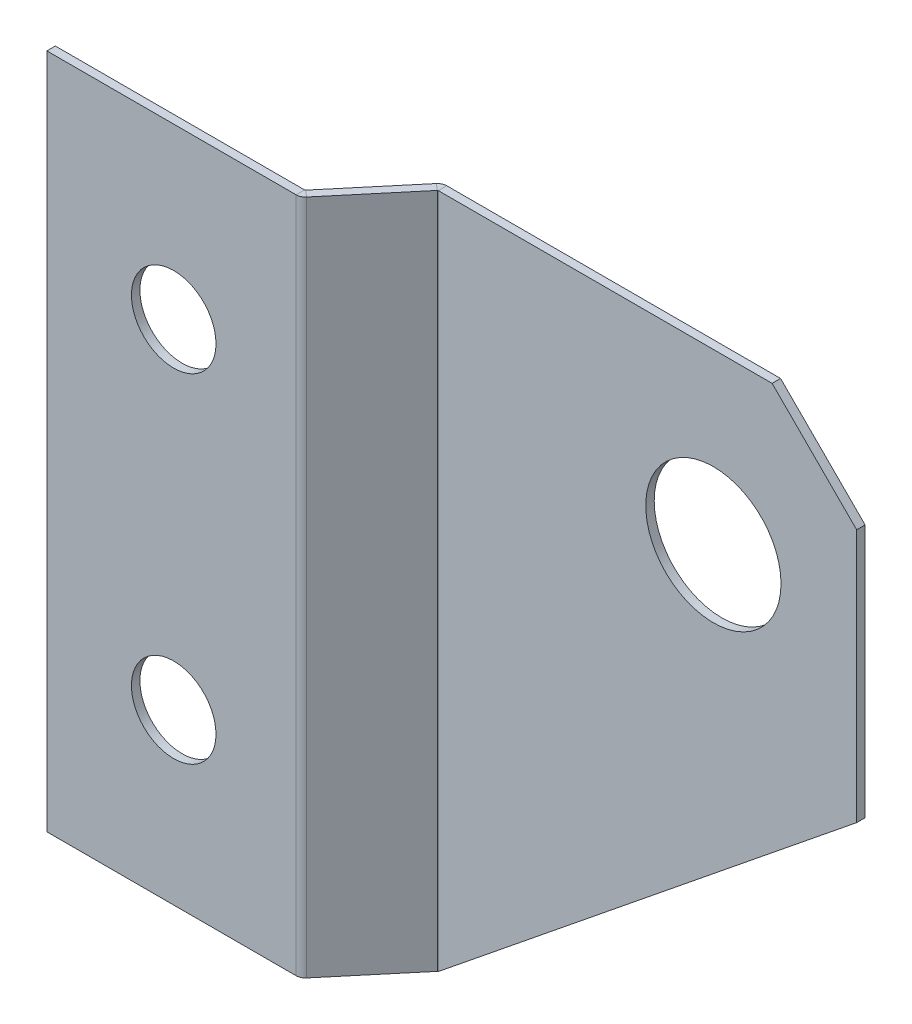
ISO-10303-21;
HEADER;
FILE_DESCRIPTION(('STEP AP214'),'2;1');
FILE_NAME('part.step','',(''),(''),'','','');
FILE_SCHEMA(('AUTOMOTIVE_DESIGN { 1 0 10303 214 1 1 1 1 }'));
ENDSEC;
DATA;
#1=APPLICATION_CONTEXT('core data for automotive mechanical design processes');
#2=APPLICATION_PROTOCOL_DEFINITION('international standard','automotive_design',2000,#1);
#3=PRODUCT_CONTEXT('',#1,'mechanical');
#4=PRODUCT('Part','Part','',(#3));
#5=PRODUCT_RELATED_PRODUCT_CATEGORY('part','',(#4));
#6=PRODUCT_DEFINITION_FORMATION('','',#4);
#7=PRODUCT_DEFINITION_CONTEXT('part definition',#1,'design');
#8=PRODUCT_DEFINITION('design','',#6,#7);
#9=PRODUCT_DEFINITION_SHAPE('','',#8);
#10=(LENGTH_UNIT() NAMED_UNIT(*) SI_UNIT(.MILLI.,.METRE.));
#11=(NAMED_UNIT(*) PLANE_ANGLE_UNIT() SI_UNIT($,.RADIAN.));
#12=(NAMED_UNIT(*) SI_UNIT($,.STERADIAN.) SOLID_ANGLE_UNIT());
#13=UNCERTAINTY_MEASURE_WITH_UNIT(LENGTH_MEASURE(1.E-05),#10,'distance_accuracy_value','');
#14=(GEOMETRIC_REPRESENTATION_CONTEXT(3) GLOBAL_UNCERTAINTY_ASSIGNED_CONTEXT((#13)) GLOBAL_UNIT_ASSIGNED_CONTEXT((#10,
#11,#12)) REPRESENTATION_CONTEXT('',''));
#15=CARTESIAN_POINT('',(0.,0.,0.));
#16=DIRECTION('',(0.,0.,1.));
#17=DIRECTION('',(1.,0.,0.));
#18=AXIS2_PLACEMENT_3D('',#15,#16,#17);
#19=CARTESIAN_POINT('',(3.85672565811926,40.,-4.59626665871385));
#20=DIRECTION('',(0.,1.,0.));
#21=DIRECTION('',(0.,0.,1.));
#22=AXIS2_PLACEMENT_3D('',#19,#20,#21);
#23=PLANE('',#22);
#24=DIRECTION('',(0.642787609686543,0.,-0.766044443118975));
#25=VECTOR('',#24,1.);
#26=CARTESIAN_POINT('',(3.85672565811926,40.,-4.59626665871385));
#27=LINE('',#26,#25);
#28=CARTESIAN_POINT('',(0.164855231730187,40.,-0.196466814672401));
#29=VERTEX_POINT('',#28);
#30=CARTESIAN_POINT('',(3.69187042638907,40.,-4.39979984404145));
#31=VERTEX_POINT('',#30);
#32=EDGE_CURVE('E239',#29,#31,#27,.T.);
#33=ORIENTED_EDGE('',*,*,#32,.T.);
#34=DIRECTION('',(-0.766044443118972,0.,-0.642787609686546));
#35=VECTOR('',#34,1.);
#36=CARTESIAN_POINT('',(3.69187042638907,40.,-4.39979984404145));
#37=LINE('',#36,#35);
#38=CARTESIAN_POINT('',(3.30884820482958,40.,-4.72119364888472));
#39=VERTEX_POINT('',#38);
#40=EDGE_CURVE('E218',#31,#39,#37,.T.);
#41=ORIENTED_EDGE('',*,*,#40,.T.);
#42=DIRECTION('',(-0.642787609686543,0.,0.766044443118975));
#43=VECTOR('',#42,1.);
#44=CARTESIAN_POINT('',(-0.479355767330552,40.,-0.20658795558327));
#45=LINE('',#44,#43);
#46=CARTESIAN_POINT('',(-0.218166989829301,40.,-0.517860619515672));
#47=VERTEX_POINT('',#46);
#48=EDGE_CURVE('E244',#47,#39,#45,.F.);
#49=ORIENTED_EDGE('',*,*,#48,.F.);
#50=DIRECTION('',(0.766044443118975,0.,0.642787609686543));
#51=VECTOR('',#50,1.);
#52=CARTESIAN_POINT('',(0.164855231730188,40.,-0.1964668146724));
#53=LINE('',#52,#51);
#54=EDGE_CURVE('E232',#47,#29,#53,.T.);
#55=ORIENTED_EDGE('',*,*,#54,.T.);
#56=EDGE_LOOP('',(#33,#41,#49,#55));
#57=FACE_BOUND('',#56,.T.);
#58=ADVANCED_FACE('F83',(#57),#23,.T.);
#59=CARTESIAN_POINT('',(-0.0963335457710638,0.,0.114805849260002));
#60=DIRECTION('',(0.766044443118975,0.,0.642787609686543));
#61=DIRECTION('',(0.642787609686543,0.,-0.766044443118975));
#62=AXIS2_PLACEMENT_3D('',#59,#60,#61);
#63=PLANE('',#62);
#64=DIRECTION('',(-0.642787609686543,0.,0.766044443118975));
#65=VECTOR('',#64,1.);
#66=CARTESIAN_POINT('',(0.149868392481989,0.,-0.178606195156728));
#67=LINE('',#66,#65);
#68=CARTESIAN_POINT('',(3.69187042638907,0.,-4.39979984404145));
#69=VERTEX_POINT('',#68);
#70=CARTESIAN_POINT('',(0.164855231730185,0.,-0.196466814672399));
#71=VERTEX_POINT('',#70);
#72=EDGE_CURVE('E240',#69,#71,#67,.T.);
#73=ORIENTED_EDGE('',*,*,#72,.F.);
#74=DIRECTION('',(0.,1.,0.));
#75=VECTOR('',#74,1.);
#76=CARTESIAN_POINT('',(3.69187042638907,40.,-4.39979984404145));
#77=LINE('',#76,#75);
#78=EDGE_CURVE('E224',#31,#69,#77,.F.);
#79=ORIENTED_EDGE('',*,*,#78,.F.);
#80=ORIENTED_EDGE('',*,*,#32,.F.);
#81=DIRECTION('',(0.,-1.,0.));
#82=VECTOR('',#81,1.);
#83=CARTESIAN_POINT('',(0.164855231730185,0.,-0.196466814672399));
#84=LINE('',#83,#82);
#85=EDGE_CURVE('E247',#29,#71,#84,.T.);
#86=ORIENTED_EDGE('',*,*,#85,.T.);
#87=EDGE_LOOP('',(#73,#79,#80,#86));
#88=FACE_BOUND('',#87,.T.);
#89=ADVANCED_FACE('F335',(#88),#63,.T.);
#90=CARTESIAN_POINT('',(-0.479355767330552,0.,-0.20658795558327));
#91=DIRECTION('',(0.766044443118975,0.,0.642787609686543));
#92=DIRECTION('',(0.642787609686543,0.,-0.766044443118975));
#93=AXIS2_PLACEMENT_3D('',#90,#91,#92);
#94=PLANE('',#93);
#95=DIRECTION('',(0.,1.,0.));
#96=VECTOR('',#95,1.);
#97=CARTESIAN_POINT('',(3.30884820482958,40.,-4.72119364888472));
#98=LINE('',#97,#96);
#99=CARTESIAN_POINT('',(3.30884820482958,0.,-4.72119364888472));
#100=VERTEX_POINT('',#99);
#101=EDGE_CURVE('E214',#39,#100,#98,.F.);
#102=ORIENTED_EDGE('',*,*,#101,.T.);
#103=DIRECTION('',(0.642787609686543,0.,-0.766044443118975));
#104=VECTOR('',#103,1.);
#105=CARTESIAN_POINT('',(-0.479355767330552,0.,-0.20658795558327));
#106=LINE('',#105,#104);
#107=CARTESIAN_POINT('',(-0.218166989829301,0.,-0.517860619515672));
#108=VERTEX_POINT('',#107);
#109=EDGE_CURVE('E243',#100,#108,#106,.F.);
#110=ORIENTED_EDGE('',*,*,#109,.T.);
#111=DIRECTION('',(0.,1.,0.));
#112=VECTOR('',#111,1.);
#113=CARTESIAN_POINT('',(-0.2181669898293,40.,-0.517860619515673));
#114=LINE('',#113,#112);
#115=EDGE_CURVE('E251',#47,#108,#114,.F.);
#116=ORIENTED_EDGE('',*,*,#115,.F.);
#117=ORIENTED_EDGE('',*,*,#48,.T.);
#118=EDGE_LOOP('',(#102,#110,#116,#117));
#119=FACE_BOUND('',#118,.T.);
#120=ADVANCED_FACE('F353',(#119),#94,.F.);
#121=CARTESIAN_POINT('',(0.,0.,-0.5));
#122=DIRECTION('',(0.,-1.,0.));
#123=DIRECTION('',(1.,0.,0.));
#124=AXIS2_PLACEMENT_3D('',#121,#122,#123);
#125=PLANE('',#124);
#126=DIRECTION('',(1.,0.,0.));
#127=VECTOR('',#126,1.);
#128=CARTESIAN_POINT('',(0.,0.,-0.5));
#129=LINE('',#128,#127);
#130=CARTESIAN_POINT('',(-15.,0.,-0.5));
#131=VERTEX_POINT('',#130);
#132=CARTESIAN_POINT('',(-0.25646921198525,0.,-0.499999999999999));
#133=VERTEX_POINT('',#132);
#134=EDGE_CURVE('E288',#131,#133,#129,.T.);
#135=ORIENTED_EDGE('',*,*,#134,.T.);
#136=DIRECTION('',(0.,0.,1.));
#137=VECTOR('',#136,1.);
#138=CARTESIAN_POINT('',(-0.25646921198525,0.,-0.499999999999999));
#139=LINE('',#138,#137);
#140=CARTESIAN_POINT('',(-0.25646921198525,0.,0.));
#141=VERTEX_POINT('',#140);
#142=EDGE_CURVE('E268',#133,#141,#139,.T.);
#143=ORIENTED_EDGE('',*,*,#142,.T.);
#144=DIRECTION('',(1.,0.,0.));
#145=VECTOR('',#144,1.);
#146=CARTESIAN_POINT('',(0.,0.,0.));
#147=LINE('',#146,#145);
#148=CARTESIAN_POINT('',(-15.,0.,0.));
#149=VERTEX_POINT('',#148);
#150=EDGE_CURVE('E285',#149,#141,#147,.T.);
#151=ORIENTED_EDGE('',*,*,#150,.F.);
#152=DIRECTION('',(0.,0.,1.));
#153=VECTOR('',#152,1.);
#154=CARTESIAN_POINT('',(-15.,0.,-0.5));
#155=LINE('',#154,#153);
#156=EDGE_CURVE('E296',#131,#149,#155,.T.);
#157=ORIENTED_EDGE('',*,*,#156,.F.);
#158=EDGE_LOOP('',(#135,#143,#151,#157));
#159=FACE_BOUND('',#158,.T.);
#160=ADVANCED_FACE('F377',(#159),#125,.T.);
#161=CARTESIAN_POINT('',(0.,0.,-0.5));
#162=DIRECTION('',(0.,0.,1.));
#163=DIRECTION('',(1.,0.,0.));
#164=AXIS2_PLACEMENT_3D('',#161,#162,#163);
#165=PLANE('',#164);
#166=CARTESIAN_POINT('',(-7.5,30.,-0.5));
#167=DIRECTION('',(0.,0.,1.));
#168=DIRECTION('',(1.,0.,0.));
#169=AXIS2_PLACEMENT_3D('',#166,#167,#168);
#170=CIRCLE('',#169,2.5);
#171=CARTESIAN_POINT('',(-5.,30.,-0.5));
#172=VERTEX_POINT('',#171);
#173=EDGE_CURVE('E639',#172,#172,#170,.T.);
#174=ORIENTED_EDGE('',*,*,#173,.T.);
#175=EDGE_LOOP('',(#174));
#176=FACE_BOUND('',#175,.T.);
#177=CARTESIAN_POINT('',(-7.5,10.,-0.5));
#178=DIRECTION('',(0.,0.,1.));
#179=DIRECTION('',(1.,0.,0.));
#180=AXIS2_PLACEMENT_3D('',#177,#178,#179);
#181=CIRCLE('',#180,2.5);
#182=CARTESIAN_POINT('',(-5.,10.,-0.5));
#183=VERTEX_POINT('',#182);
#184=EDGE_CURVE('E650',#183,#183,#181,.T.);
#185=ORIENTED_EDGE('',*,*,#184,.T.);
#186=EDGE_LOOP('',(#185));
#187=FACE_BOUND('',#186,.T.);
#188=DIRECTION('',(0.,-1.,0.));
#189=VECTOR('',#188,1.);
#190=CARTESIAN_POINT('',(-0.25646921198525,0.,-0.499999999999999));
#191=LINE('',#190,#189);
#192=CARTESIAN_POINT('',(-0.25646921198525,40.,-0.499999999999999));
#193=VERTEX_POINT('',#192);
#194=EDGE_CURVE('E275',#133,#193,#191,.F.);
#195=ORIENTED_EDGE('',*,*,#194,.F.);
#196=ORIENTED_EDGE('',*,*,#134,.F.);
#197=DIRECTION('',(0.,-1.,0.));
#198=VECTOR('',#197,1.);
#199=CARTESIAN_POINT('',(-15.,0.,-0.5));
#200=LINE('',#199,#198);
#201=CARTESIAN_POINT('',(-15.,40.,-0.5));
#202=VERTEX_POINT('',#201);
#203=EDGE_CURVE('E283',#202,#131,#200,.T.);
#204=ORIENTED_EDGE('',*,*,#203,.F.);
#205=DIRECTION('',(-1.,0.,0.));
#206=VECTOR('',#205,1.);
#207=CARTESIAN_POINT('',(0.,40.,-0.5));
#208=LINE('',#207,#206);
#209=EDGE_CURVE('E282',#193,#202,#208,.T.);
#210=ORIENTED_EDGE('',*,*,#209,.F.);
#211=EDGE_LOOP('',(#195,#196,#204,#210));
#212=FACE_BOUND('',#211,.T.);
#213=ADVANCED_FACE('F372',(#176,#187,#212),#165,.F.);
#214=CARTESIAN_POINT('',(0.,0.,0.));
#215=DIRECTION('',(0.,0.,1.));
#216=DIRECTION('',(1.,0.,0.));
#217=AXIS2_PLACEMENT_3D('',#214,#215,#216);
#218=PLANE('',#217);
#219=CARTESIAN_POINT('',(-7.5,30.,0.));
#220=DIRECTION('',(0.,0.,1.));
#221=DIRECTION('',(1.,0.,0.));
#222=AXIS2_PLACEMENT_3D('',#219,#220,#221);
#223=CIRCLE('',#222,2.5);
#224=CARTESIAN_POINT('',(-5.,30.,0.));
#225=VERTEX_POINT('',#224);
#226=EDGE_CURVE('E648',#225,#225,#223,.T.);
#227=ORIENTED_EDGE('',*,*,#226,.F.);
#228=EDGE_LOOP('',(#227));
#229=FACE_BOUND('',#228,.T.);
#230=CARTESIAN_POINT('',(-7.5,10.,0.));
#231=DIRECTION('',(0.,0.,1.));
#232=DIRECTION('',(1.,0.,0.));
#233=AXIS2_PLACEMENT_3D('',#230,#231,#232);
#234=CIRCLE('',#233,2.5);
#235=CARTESIAN_POINT('',(-5.,10.,0.));
#236=VERTEX_POINT('',#235);
#237=EDGE_CURVE('E653',#236,#236,#234,.T.);
#238=ORIENTED_EDGE('',*,*,#237,.F.);
#239=EDGE_LOOP('',(#238));
#240=FACE_BOUND('',#239,.T.);
#241=ORIENTED_EDGE('',*,*,#150,.T.);
#242=DIRECTION('',(0.,-1.,0.));
#243=VECTOR('',#242,1.);
#244=CARTESIAN_POINT('',(-0.25646921198525,0.,0.));
#245=LINE('',#244,#243);
#246=CARTESIAN_POINT('',(-0.25646921198525,40.,0.));
#247=VERTEX_POINT('',#246);
#248=EDGE_CURVE('E256',#141,#247,#245,.F.);
#249=ORIENTED_EDGE('',*,*,#248,.T.);
#250=DIRECTION('',(-1.,0.,0.));
#251=VECTOR('',#250,1.);
#252=CARTESIAN_POINT('',(0.,40.,0.));
#253=LINE('',#252,#251);
#254=CARTESIAN_POINT('',(-15.,40.,0.));
#255=VERTEX_POINT('',#254);
#256=EDGE_CURVE('E276',#247,#255,#253,.T.);
#257=ORIENTED_EDGE('',*,*,#256,.T.);
#258=DIRECTION('',(0.,-1.,0.));
#259=VECTOR('',#258,1.);
#260=CARTESIAN_POINT('',(-15.,0.,0.));
#261=LINE('',#260,#259);
#262=EDGE_CURVE('E291',#255,#149,#261,.T.);
#263=ORIENTED_EDGE('',*,*,#262,.T.);
#264=EDGE_LOOP('',(#241,#249,#257,#263));
#265=FACE_BOUND('',#264,.T.);
#266=ADVANCED_FACE('F380',(#229,#240,#265),#218,.T.);
#267=CARTESIAN_POINT('',(-15.,0.,-0.5));
#268=DIRECTION('',(-1.,0.,0.));
#269=DIRECTION('',(0.,-1.,0.));
#270=AXIS2_PLACEMENT_3D('',#267,#268,#269);
#271=PLANE('',#270);
#272=ORIENTED_EDGE('',*,*,#262,.F.);
#273=DIRECTION('',(0.,0.,1.));
#274=VECTOR('',#273,1.);
#275=CARTESIAN_POINT('',(-15.,40.,-0.5));
#276=LINE('',#275,#274);
#277=EDGE_CURVE('E293',#202,#255,#276,.T.);
#278=ORIENTED_EDGE('',*,*,#277,.F.);
#279=ORIENTED_EDGE('',*,*,#203,.T.);
#280=ORIENTED_EDGE('',*,*,#156,.T.);
#281=EDGE_LOOP('',(#272,#278,#279,#280));
#282=FACE_BOUND('',#281,.T.);
#283=ADVANCED_FACE('F385',(#282),#271,.T.);
#284=CARTESIAN_POINT('',(0.,40.,-0.5));
#285=DIRECTION('',(0.,1.,0.));
#286=DIRECTION('',(0.,0.,1.));
#287=AXIS2_PLACEMENT_3D('',#284,#285,#286);
#288=PLANE('',#287);
#289=DIRECTION('',(0.,0.,1.));
#290=VECTOR('',#289,1.);
#291=CARTESIAN_POINT('',(-0.25646921198525,40.,-0.499999999999999));
#292=LINE('',#291,#290);
#293=EDGE_CURVE('E277',#193,#247,#292,.T.);
#294=ORIENTED_EDGE('',*,*,#293,.F.);
#295=ORIENTED_EDGE('',*,*,#209,.T.);
#296=ORIENTED_EDGE('',*,*,#277,.T.);
#297=ORIENTED_EDGE('',*,*,#256,.F.);
#298=EDGE_LOOP('',(#294,#295,#296,#297));
#299=FACE_BOUND('',#298,.T.);
#300=ADVANCED_FACE('F367',(#299),#288,.T.);
#301=CARTESIAN_POINT('',(-0.25646921198525,40.,-0.549999999999999));
#302=DIRECTION('',(0.,1.,0.));
#303=DIRECTION('',(0.,0.,1.));
#304=AXIS2_PLACEMENT_3D('',#301,#302,#303);
#305=PLANE('',#304);
#306=ORIENTED_EDGE('',*,*,#54,.F.);
#307=CARTESIAN_POINT('',(-0.25646921198525,40.,-0.549999999999999));
#308=DIRECTION('',(0.,-1.,0.));
#309=DIRECTION('',(0.,0.,-1.));
#310=AXIS2_PLACEMENT_3D('',#307,#308,#309);
#311=CIRCLE('',#310,0.0500000000000002);
#312=EDGE_CURVE('E269',#193,#47,#311,.F.);
#313=ORIENTED_EDGE('',*,*,#312,.F.);
#314=ORIENTED_EDGE('',*,*,#293,.T.);
#315=CARTESIAN_POINT('',(-0.25646921198525,40.,-0.549999999999999));
#316=DIRECTION('',(0.,-1.,0.));
#317=DIRECTION('',(0.,0.,-1.));
#318=AXIS2_PLACEMENT_3D('',#315,#316,#317);
#319=CIRCLE('',#318,0.55);
#320=EDGE_CURVE('E265',#247,#29,#319,.F.);
#321=ORIENTED_EDGE('',*,*,#320,.T.);
#322=EDGE_LOOP('',(#306,#313,#314,#321));
#323=FACE_BOUND('',#322,.T.);
#324=ADVANCED_FACE('F366',(#323),#305,.T.);
#325=CARTESIAN_POINT('',(-0.25646921198525,0.,-0.549999999999999));
#326=DIRECTION('',(0.,1.,0.));
#327=DIRECTION('',(0.,0.,1.));
#328=AXIS2_PLACEMENT_3D('',#325,#326,#327);
#329=PLANE('',#328);
#330=CARTESIAN_POINT('',(-0.25646921198525,0.,-0.549999999999999));
#331=DIRECTION('',(0.,-1.,0.));
#332=DIRECTION('',(0.,0.,-1.));
#333=AXIS2_PLACEMENT_3D('',#330,#331,#332);
#334=CIRCLE('',#333,0.0500000000000002);
#335=EDGE_CURVE('E237',#108,#133,#334,.T.);
#336=ORIENTED_EDGE('',*,*,#335,.F.);
#337=DIRECTION('',(0.766044443118975,0.,0.642787609686543));
#338=VECTOR('',#337,1.);
#339=CARTESIAN_POINT('',(-0.218166989829302,0.,-0.51786061951567));
#340=LINE('',#339,#338);
#341=EDGE_CURVE('E252',#108,#71,#340,.T.);
#342=ORIENTED_EDGE('',*,*,#341,.T.);
#343=CARTESIAN_POINT('',(-0.25646921198525,0.,-0.549999999999999));
#344=DIRECTION('',(0.,-1.,0.));
#345=DIRECTION('',(0.,0.,-1.));
#346=AXIS2_PLACEMENT_3D('',#343,#344,#345);
#347=CIRCLE('',#346,0.55);
#348=EDGE_CURVE('E261',#71,#141,#347,.T.);
#349=ORIENTED_EDGE('',*,*,#348,.T.);
#350=ORIENTED_EDGE('',*,*,#142,.F.);
#351=EDGE_LOOP('',(#336,#342,#349,#350));
#352=FACE_BOUND('',#351,.T.);
#353=ADVANCED_FACE('F365',(#352),#329,.F.);
#354=CARTESIAN_POINT('',(-0.25646921198525,0.,-0.549999999999999));
#355=DIRECTION('',(0.,-1.,0.));
#356=DIRECTION('',(0.766044443118975,0.,0.642787609686543));
#357=AXIS2_PLACEMENT_3D('',#354,#355,#356);
#358=CYLINDRICAL_SURFACE('',#357,0.55);
#359=ORIENTED_EDGE('',*,*,#248,.F.);
#360=ORIENTED_EDGE('',*,*,#348,.F.);
#361=ORIENTED_EDGE('',*,*,#85,.F.);
#362=ORIENTED_EDGE('',*,*,#320,.F.);
#363=EDGE_LOOP('',(#359,#360,#361,#362));
#364=FACE_BOUND('',#363,.T.);
#365=ADVANCED_FACE('F356',(#364),#358,.T.);
#366=CARTESIAN_POINT('',(-0.25646921198525,0.,-0.549999999999999));
#367=DIRECTION('',(0.,-1.,0.));
#368=DIRECTION('',(0.766044443118975,0.,0.642787609686543));
#369=AXIS2_PLACEMENT_3D('',#366,#367,#368);
#370=CYLINDRICAL_SURFACE('',#369,0.0500000000000002);
#371=ORIENTED_EDGE('',*,*,#194,.T.);
#372=ORIENTED_EDGE('',*,*,#312,.T.);
#373=ORIENTED_EDGE('',*,*,#115,.T.);
#374=ORIENTED_EDGE('',*,*,#335,.T.);
#375=EDGE_LOOP('',(#371,#372,#373,#374));
#376=FACE_BOUND('',#375,.T.);
#377=ADVANCED_FACE('F363',(#376),#370,.F.);
#378=CARTESIAN_POINT('',(0.149868392481989,0.,-0.178606195156728));
#379=DIRECTION('',(0.,-1.,0.));
#380=DIRECTION('',(0.,0.,-1.));
#381=AXIS2_PLACEMENT_3D('',#378,#379,#380);
#382=PLANE('',#381);
#383=DIRECTION('',(-0.766044443118972,0.,-0.642787609686546));
#384=VECTOR('',#383,1.);
#385=CARTESIAN_POINT('',(3.69187042638907,0.,-4.39979984404145));
#386=LINE('',#385,#384);
#387=EDGE_CURVE('E235',#69,#100,#386,.T.);
#388=ORIENTED_EDGE('',*,*,#387,.F.);
#389=ORIENTED_EDGE('',*,*,#72,.T.);
#390=ORIENTED_EDGE('',*,*,#341,.F.);
#391=ORIENTED_EDGE('',*,*,#109,.F.);
#392=EDGE_LOOP('',(#388,#389,#390,#391));
#393=FACE_BOUND('',#392,.T.);
#394=ADVANCED_FACE('F326',(#393),#382,.T.);
#395=CARTESIAN_POINT('',(3.73017264854502,0.,-4.36766046355712));
#396=DIRECTION('',(0.,-1.,0.));
#397=DIRECTION('',(0.,0.,-1.));
#398=AXIS2_PLACEMENT_3D('',#395,#396,#397);
#399=PLANE('',#398);
#400=DIRECTION('',(0.,0.,-1.));
#401=VECTOR('',#400,1.);
#402=CARTESIAN_POINT('',(3.73017264854501,0.,-4.91766046355715));
#403=LINE('',#402,#401);
#404=CARTESIAN_POINT('',(3.73017264854502,0.,-4.41766046355712));
#405=VERTEX_POINT('',#404);
#406=CARTESIAN_POINT('',(3.73017264854502,0.,-4.91766046355713));
#407=VERTEX_POINT('',#406);
#408=EDGE_CURVE('E212',#405,#407,#403,.T.);
#409=ORIENTED_EDGE('',*,*,#408,.F.);
#410=CARTESIAN_POINT('',(3.73017264854502,0.,-4.36766046355712));
#411=DIRECTION('',(0.,1.,0.));
#412=DIRECTION('',(0.,0.,1.));
#413=AXIS2_PLACEMENT_3D('',#410,#411,#412);
#414=CIRCLE('',#413,0.0500000000000006);
#415=EDGE_CURVE('E225',#69,#405,#414,.F.);
#416=ORIENTED_EDGE('',*,*,#415,.F.);
#417=ORIENTED_EDGE('',*,*,#387,.T.);
#418=CARTESIAN_POINT('',(3.73017264854502,0.,-4.36766046355712));
#419=DIRECTION('',(0.,1.,0.));
#420=DIRECTION('',(0.,0.,1.));
#421=AXIS2_PLACEMENT_3D('',#418,#419,#420);
#422=CIRCLE('',#421,0.550000000000001);
#423=EDGE_CURVE('E213',#100,#407,#422,.F.);
#424=ORIENTED_EDGE('',*,*,#423,.T.);
#425=EDGE_LOOP('',(#409,#416,#417,#424));
#426=FACE_BOUND('',#425,.T.);
#427=ADVANCED_FACE('F324',(#426),#399,.T.);
#428=CARTESIAN_POINT('',(3.73017264854502,40.,-4.36766046355712));
#429=DIRECTION('',(0.,-1.,0.));
#430=DIRECTION('',(0.,0.,-1.));
#431=AXIS2_PLACEMENT_3D('',#428,#429,#430);
#432=PLANE('',#431);
#433=CARTESIAN_POINT('',(3.73017264854502,40.,-4.36766046355712));
#434=DIRECTION('',(0.,1.,0.));
#435=DIRECTION('',(0.,0.,1.));
#436=AXIS2_PLACEMENT_3D('',#433,#434,#435);
#437=CIRCLE('',#436,0.0500000000000006);
#438=CARTESIAN_POINT('',(3.73017264854502,40.,-4.41766046355712));
#439=VERTEX_POINT('',#438);
#440=EDGE_CURVE('E226',#439,#31,#437,.T.);
#441=ORIENTED_EDGE('',*,*,#440,.F.);
#442=DIRECTION('',(0.,0.,-1.));
#443=VECTOR('',#442,1.);
#444=CARTESIAN_POINT('',(3.73017264854502,40.,-4.41766046355712));
#445=LINE('',#444,#443);
#446=CARTESIAN_POINT('',(3.73017264854502,40.,-4.91766046355712));
#447=VERTEX_POINT('',#446);
#448=EDGE_CURVE('E204',#439,#447,#445,.T.);
#449=ORIENTED_EDGE('',*,*,#448,.T.);
#450=CARTESIAN_POINT('',(3.73017264854502,40.,-4.36766046355712));
#451=DIRECTION('',(0.,1.,0.));
#452=DIRECTION('',(0.,0.,1.));
#453=AXIS2_PLACEMENT_3D('',#450,#451,#452);
#454=CIRCLE('',#453,0.550000000000001);
#455=EDGE_CURVE('E216',#447,#39,#454,.T.);
#456=ORIENTED_EDGE('',*,*,#455,.T.);
#457=ORIENTED_EDGE('',*,*,#40,.F.);
#458=EDGE_LOOP('',(#441,#449,#456,#457));
#459=FACE_BOUND('',#458,.T.);
#460=ADVANCED_FACE('F314',(#459),#432,.F.);
#461=CARTESIAN_POINT('',(3.73017264854502,40.,-4.36766046355712));
#462=DIRECTION('',(0.,1.,0.));
#463=DIRECTION('',(0.,0.,-1.));
#464=AXIS2_PLACEMENT_3D('',#461,#462,#463);
#465=CYLINDRICAL_SURFACE('',#464,0.550000000000001);
#466=ORIENTED_EDGE('',*,*,#101,.F.);
#467=ORIENTED_EDGE('',*,*,#455,.F.);
#468=DIRECTION('',(0.,1.,0.));
#469=VECTOR('',#468,1.);
#470=CARTESIAN_POINT('',(3.73017264854501,0.,-4.91766046355712));
#471=LINE('',#470,#469);
#472=EDGE_CURVE('E199',#407,#447,#471,.T.);
#473=ORIENTED_EDGE('',*,*,#472,.F.);
#474=ORIENTED_EDGE('',*,*,#423,.F.);
#475=EDGE_LOOP('',(#466,#467,#473,#474));
#476=FACE_BOUND('',#475,.T.);
#477=ADVANCED_FACE('F322',(#476),#465,.T.);
#478=CARTESIAN_POINT('',(3.73017264854502,40.,-4.36766046355712));
#479=DIRECTION('',(0.,1.,0.));
#480=DIRECTION('',(0.,0.,-1.));
#481=AXIS2_PLACEMENT_3D('',#478,#479,#480);
#482=CYLINDRICAL_SURFACE('',#481,0.0500000000000006);
#483=ORIENTED_EDGE('',*,*,#78,.T.);
#484=ORIENTED_EDGE('',*,*,#415,.T.);
#485=DIRECTION('',(0.,-1.,0.));
#486=VECTOR('',#485,1.);
#487=CARTESIAN_POINT('',(3.73017264854501,0.,-4.41766046355712));
#488=LINE('',#487,#486);
#489=EDGE_CURVE('E192',#405,#439,#488,.F.);
#490=ORIENTED_EDGE('',*,*,#489,.T.);
#491=ORIENTED_EDGE('',*,*,#440,.T.);
#492=EDGE_LOOP('',(#483,#484,#490,#491));
#493=FACE_BOUND('',#492,.T.);
#494=ADVANCED_FACE('F332',(#493),#482,.F.);
#495=CARTESIAN_POINT('',(3.70685726563726,40.,-4.91766046355712));
#496=DIRECTION('',(0.,1.,0.));
#497=DIRECTION('',(0.,0.,1.));
#498=AXIS2_PLACEMENT_3D('',#495,#496,#497);
#499=PLANE('',#498);
#500=DIRECTION('',(1.,0.,0.));
#501=VECTOR('',#500,1.);
#502=CARTESIAN_POINT('',(-0.149868392481995,40.,-4.41766046355712));
#503=LINE('',#502,#501);
#504=CARTESIAN_POINT('',(23.4737034365597,40.,-4.41766046355714));
#505=VERTEX_POINT('',#504);
#506=EDGE_CURVE('E196',#505,#439,#503,.F.);
#507=ORIENTED_EDGE('',*,*,#506,.F.);
#508=DIRECTION('',(0.,0.,-1.));
#509=VECTOR('',#508,1.);
#510=CARTESIAN_POINT('',(23.4737034365597,40.,-4.91766046355714));
#511=LINE('',#510,#509);
#512=CARTESIAN_POINT('',(23.4737034365597,40.,-4.91766046355714));
#513=VERTEX_POINT('',#512);
#514=EDGE_CURVE('E108',#505,#513,#511,.T.);
#515=ORIENTED_EDGE('',*,*,#514,.T.);
#516=DIRECTION('',(-1.,0.,0.));
#517=VECTOR('',#516,1.);
#518=CARTESIAN_POINT('',(3.70685726563726,40.,-4.91766046355712));
#519=LINE('',#518,#517);
#520=EDGE_CURVE('E233',#513,#447,#519,.T.);
#521=ORIENTED_EDGE('',*,*,#520,.T.);
#522=ORIENTED_EDGE('',*,*,#448,.F.);
#523=EDGE_LOOP('',(#507,#515,#521,#522));
#524=FACE_BOUND('',#523,.T.);
#525=ADVANCED_FACE('F311',(#524),#499,.T.);
#526=CARTESIAN_POINT('',(-0.149868392481995,0.,-4.91766046355712));
#527=DIRECTION('',(0.,0.,-1.));
#528=DIRECTION('',(-1.,0.,0.));
#529=AXIS2_PLACEMENT_3D('',#526,#527,#528);
#530=PLANE('',#529);
#531=CARTESIAN_POINT('',(20.,30.,-4.91766046355714));
#532=DIRECTION('',(0.,0.,-1.));
#533=DIRECTION('',(-1.,0.,0.));
#534=AXIS2_PLACEMENT_3D('',#531,#532,#533);
#535=CIRCLE('',#534,4.);
#536=CARTESIAN_POINT('',(16.,30.,-4.91766046355713));
#537=VERTEX_POINT('',#536);
#538=EDGE_CURVE('E195',#537,#537,#535,.T.);
#539=ORIENTED_EDGE('',*,*,#538,.F.);
#540=EDGE_LOOP('',(#539));
#541=FACE_BOUND('',#540,.T.);
#542=DIRECTION('',(0.77771312299015,0.628619358856302,0.));
#543=VECTOR('',#542,1.);
#544=CARTESIAN_POINT('',(1.38337754290073,-1.89689590038704,-4.91766046355712));
#545=LINE('',#544,#543);
#546=CARTESIAN_POINT('',(28.4737034365598,20.,-4.91766046355715));
#547=VERTEX_POINT('',#546);
#548=EDGE_CURVE('E99',#407,#547,#545,.T.);
#549=ORIENTED_EDGE('',*,*,#548,.F.);
#550=ORIENTED_EDGE('',*,*,#472,.T.);
#551=ORIENTED_EDGE('',*,*,#520,.F.);
#552=DIRECTION('',(-0.70710678118655,0.707106781186546,0.));
#553=VECTOR('',#552,1.);
#554=CARTESIAN_POINT('',(31.6619175220388,31.811785914521,-4.91766046355715));
#555=LINE('',#554,#553);
#556=CARTESIAN_POINT('',(28.4737034365598,35.,-4.91766046355715));
#557=VERTEX_POINT('',#556);
#558=EDGE_CURVE('E92',#513,#557,#555,.F.);
#559=ORIENTED_EDGE('',*,*,#558,.T.);
#560=DIRECTION('',(0.,1.,0.));
#561=VECTOR('',#560,1.);
#562=CARTESIAN_POINT('',(28.4737034365598,40.,-4.91766046355715));
#563=LINE('',#562,#561);
#564=EDGE_CURVE('E203',#547,#557,#563,.T.);
#565=ORIENTED_EDGE('',*,*,#564,.F.);
#566=EDGE_LOOP('',(#549,#550,#551,#559,#565));
#567=FACE_BOUND('',#566,.T.);
#568=ADVANCED_FACE('F308',(#541,#567),#530,.T.);
#569=CARTESIAN_POINT('',(-0.149868392481995,0.,-4.41766046355712));
#570=DIRECTION('',(0.,0.,-1.));
#571=DIRECTION('',(-1.,0.,0.));
#572=AXIS2_PLACEMENT_3D('',#569,#570,#571);
#573=PLANE('',#572);
#574=CARTESIAN_POINT('',(20.,30.,-4.41766046355712));
#575=DIRECTION('',(0.,0.,1.));
#576=DIRECTION('',(1.,0.,0.));
#577=AXIS2_PLACEMENT_3D('',#574,#575,#576);
#578=CIRCLE('',#577,4.);
#579=CARTESIAN_POINT('',(24.,30.,-4.41766046355712));
#580=VERTEX_POINT('',#579);
#581=EDGE_CURVE('E640',#580,#580,#578,.T.);
#582=ORIENTED_EDGE('',*,*,#581,.F.);
#583=EDGE_LOOP('',(#582));
#584=FACE_BOUND('',#583,.T.);
#585=ORIENTED_EDGE('',*,*,#489,.F.);
#586=DIRECTION('',(-0.77771312299015,-0.628619358856302,0.));
#587=VECTOR('',#586,1.);
#588=CARTESIAN_POINT('',(3.73017264854502,0.,-4.41766046355712));
#589=LINE('',#588,#587);
#590=CARTESIAN_POINT('',(28.4737034365598,20.,-4.41766046355712));
#591=VERTEX_POINT('',#590);
#592=EDGE_CURVE('E179',#591,#405,#589,.T.);
#593=ORIENTED_EDGE('',*,*,#592,.F.);
#594=DIRECTION('',(0.,-1.,0.));
#595=VECTOR('',#594,1.);
#596=CARTESIAN_POINT('',(28.4737034365598,0.,-4.41766046355715));
#597=LINE('',#596,#595);
#598=CARTESIAN_POINT('',(28.4737034365598,35.,-4.41766046355715));
#599=VERTEX_POINT('',#598);
#600=EDGE_CURVE('E189',#591,#599,#597,.F.);
#601=ORIENTED_EDGE('',*,*,#600,.T.);
#602=DIRECTION('',(0.70710678118655,-0.707106781186546,0.));
#603=VECTOR('',#602,1.);
#604=CARTESIAN_POINT('',(28.4737034365598,35.,-4.41766046355715));
#605=LINE('',#604,#603);
#606=EDGE_CURVE('E303',#599,#505,#605,.F.);
#607=ORIENTED_EDGE('',*,*,#606,.T.);
#608=ORIENTED_EDGE('',*,*,#506,.T.);
#609=EDGE_LOOP('',(#585,#593,#601,#607,#608));
#610=FACE_BOUND('',#609,.T.);
#611=ADVANCED_FACE('F190',(#584,#610),#573,.F.);
#612=CARTESIAN_POINT('',(28.4737034365598,40.,-4.91766046355715));
#613=DIRECTION('',(1.,0.,0.));
#614=DIRECTION('',(0.,0.,-1.));
#615=AXIS2_PLACEMENT_3D('',#612,#613,#614);
#616=PLANE('',#615);
#617=DIRECTION('',(0.,0.,1.));
#618=VECTOR('',#617,1.);
#619=CARTESIAN_POINT('',(28.4737034365598,20.,-4.91766046355713));
#620=LINE('',#619,#618);
#621=EDGE_CURVE('E13',#547,#591,#620,.T.);
#622=ORIENTED_EDGE('',*,*,#621,.F.);
#623=ORIENTED_EDGE('',*,*,#564,.T.);
#624=DIRECTION('',(0.,0.,1.));
#625=VECTOR('',#624,1.);
#626=CARTESIAN_POINT('',(28.4737034365598,35.,-4.91766046355715));
#627=LINE('',#626,#625);
#628=EDGE_CURVE('E200',#557,#599,#627,.T.);
#629=ORIENTED_EDGE('',*,*,#628,.T.);
#630=ORIENTED_EDGE('',*,*,#600,.F.);
#631=EDGE_LOOP('',(#622,#623,#629,#630));
#632=FACE_BOUND('',#631,.T.);
#633=ADVANCED_FACE('F193',(#632),#616,.T.);
#634=CARTESIAN_POINT('',(28.4737034365598,35.,-4.91766046355715));
#635=DIRECTION('',(-0.707106781186546,-0.70710678118655,0.));
#636=DIRECTION('',(0.,0.,1.));
#637=AXIS2_PLACEMENT_3D('',#634,#635,#636);
#638=PLANE('',#637);
#639=ORIENTED_EDGE('',*,*,#558,.F.);
#640=ORIENTED_EDGE('',*,*,#514,.F.);
#641=ORIENTED_EDGE('',*,*,#606,.F.);
#642=ORIENTED_EDGE('',*,*,#628,.F.);
#643=EDGE_LOOP('',(#639,#640,#641,#642));
#644=FACE_BOUND('',#643,.T.);
#645=ADVANCED_FACE('F89',(#644),#638,.F.);
#646=CARTESIAN_POINT('',(3.73017264854502,0.,-14.4176604635571));
#647=DIRECTION('',(-0.628619358856302,0.77771312299015,0.));
#648=DIRECTION('',(-0.77771312299015,-0.628619358856302,0.));
#649=AXIS2_PLACEMENT_3D('',#646,#647,#648);
#650=PLANE('',#649);
#651=ORIENTED_EDGE('',*,*,#548,.T.);
#652=ORIENTED_EDGE('',*,*,#621,.T.);
#653=ORIENTED_EDGE('',*,*,#592,.T.);
#654=ORIENTED_EDGE('',*,*,#408,.T.);
#655=EDGE_LOOP('',(#651,#652,#653,#654));
#656=FACE_BOUND('',#655,.T.);
#657=ADVANCED_FACE('F177',(#656),#650,.F.);
#658=CARTESIAN_POINT('',(20.,30.,-14.4176604635571));
#659=DIRECTION('',(0.,0.,1.));
#660=DIRECTION('',(1.,0.,0.));
#661=AXIS2_PLACEMENT_3D('',#658,#659,#660);
#662=CYLINDRICAL_SURFACE('',#661,4.);
#663=ORIENTED_EDGE('',*,*,#538,.T.);
#664=EDGE_LOOP('',(#663));
#665=FACE_BOUND('',#664,.T.);
#666=ORIENTED_EDGE('',*,*,#581,.T.);
#667=EDGE_LOOP('',(#666));
#668=FACE_BOUND('',#667,.T.);
#669=ADVANCED_FACE('F453',(#665,#668),#662,.F.);
#670=CARTESIAN_POINT('',(-7.5,10.,-10.));
#671=DIRECTION('',(0.,0.,1.));
#672=DIRECTION('',(1.,0.,0.));
#673=AXIS2_PLACEMENT_3D('',#670,#671,#672);
#674=CYLINDRICAL_SURFACE('',#673,2.5);
#675=ORIENTED_EDGE('',*,*,#237,.T.);
#676=EDGE_LOOP('',(#675));
#677=FACE_BOUND('',#676,.T.);
#678=ORIENTED_EDGE('',*,*,#184,.F.);
#679=EDGE_LOOP('',(#678));
#680=FACE_BOUND('',#679,.T.);
#681=ADVANCED_FACE('F467',(#677,#680),#674,.F.);
#682=CARTESIAN_POINT('',(-7.5,30.,-10.));
#683=DIRECTION('',(0.,0.,1.));
#684=DIRECTION('',(1.,0.,0.));
#685=AXIS2_PLACEMENT_3D('',#682,#683,#684);
#686=CYLINDRICAL_SURFACE('',#685,2.5);
#687=ORIENTED_EDGE('',*,*,#226,.T.);
#688=EDGE_LOOP('',(#687));
#689=FACE_BOUND('',#688,.T.);
#690=ORIENTED_EDGE('',*,*,#173,.F.);
#691=EDGE_LOOP('',(#690));
#692=FACE_BOUND('',#691,.T.);
#693=ADVANCED_FACE('F479',(#689,#692),#686,.F.);
#694=CLOSED_SHELL('',(#58,#89,#120,#160,#213,#266,#283,#300,#324,#353,#365,#377,#394,#427,#460,
#477,#494,#525,#568,#611,#633,#645,#657,#669,#681,#693));
#695=MANIFOLD_SOLID_BREP('B2',#694);
#696=ADVANCED_BREP_SHAPE_REPRESENTATION('',(#18,#695),#14);
#697=SHAPE_DEFINITION_REPRESENTATION(#9,#696);
ENDSEC;
END-ISO-10303-21;
